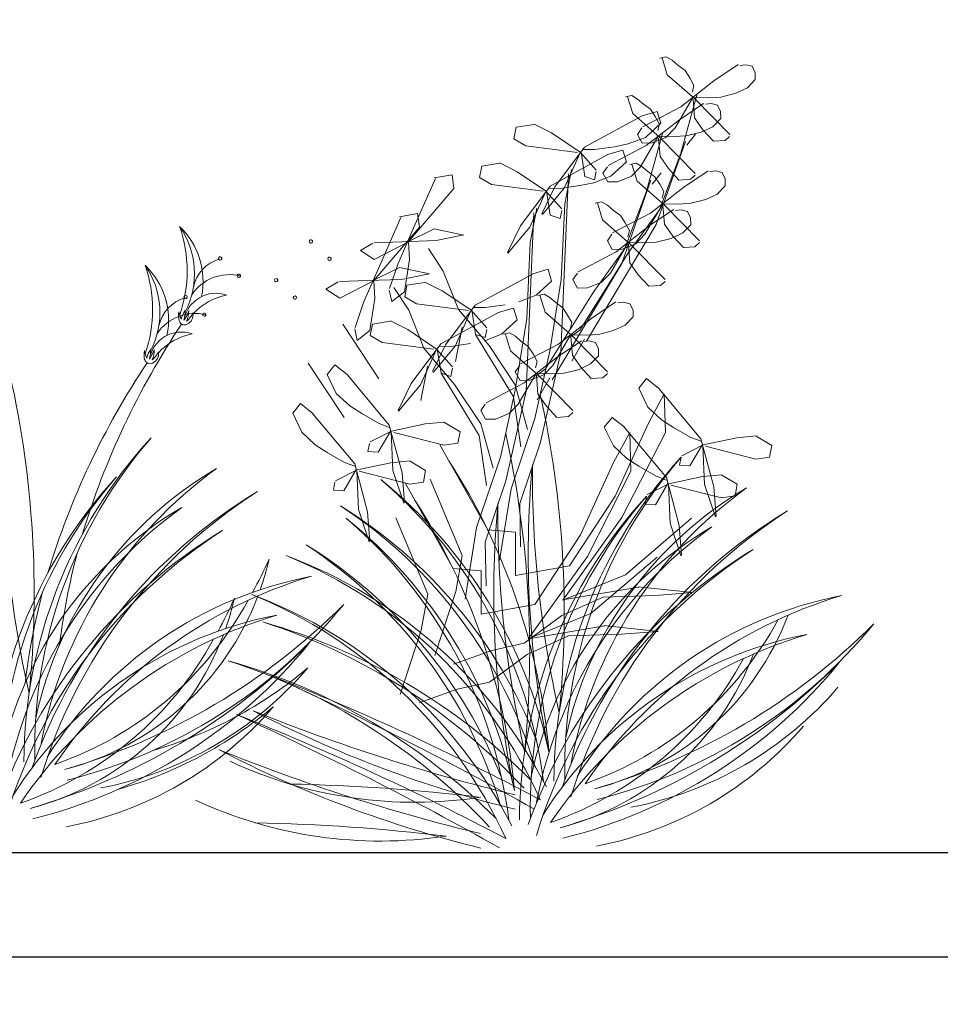
# Model space of a CAD drawing. Units: inches. Extents: x 89 to 490, y -59 to 378.
# Tile 14 of 20: x 400 to 429, y -28 to 3. Entities that reach past the tile are written whole.
import ezdxf

# ---------------------------------------------------------------- set-up
doc = ezdxf.new("R2010")
doc.units = ezdxf.units.IN
doc.header["$MEASUREMENT"] = 0
for name, color, linetype, lineweight in [('A-ANNO-DIMS', 2, 'Continuous', 18), ('L-PLNT', 94, 'Continuous', 18), ('L-PLNT-EDGE', 31, 'Continuous', 25)]:
    doc.layers.add(name, color=color, linetype=linetype, lineweight=lineweight)
doc.layers.add('fl', color=73, linetype='Continuous', lineweight=9, true_color=0xa3d166)
doc.styles.get("Standard").update_dxf_attribs({"font": 'arial.ttf'})
doc.dimstyles.get("Standard").update_dxf_attribs({"dimtxt": 6, "dimasz": 4, "dimexe": 3, "dimexo": 3, "dimgap": 0.09, "dimtad": 0, "dimtih": 1, "dimtoh": 1, "dimdec": 1, "dimzin": 0, "dimdsep": 46, "dimlunit": 3, "dimtxsty": 'Standard', "dimcen": 0.09, "dimadec": 0, "dimazin": 0, "dimtfac": 1, "dimtdec": 1, "dimtofl": 0, "dimtmove": 0, "dimatfit": 3, "dimfxl": 1, "dimtolj": 1, "dimtzin": 0, "dimarcsym": 0})

# ---------------------------------------------------------------- blocks, each defined once
blk = doc.blocks.new('Plantation')
at = {"layer": 'fl'}
for p, q in [((644.446, 36.432), (644.645, 36.472)), ((644.513, 36.439), (644.677, 35.91)), ((644.645, 36.472), (644.829, 36.366)), ((644.829, 36.366), (645.013, 36.206)), ((645.013, 36.206), (645.235, 36.046)), ((646.142, 35.717), (646.902, 36.229)), ((647.142, 36.225), (646.96, 36.203)), ((647.343, 36.174), (647.142, 36.225)), ((647.437, 35.975), (647.343, 36.174)), ((644.677, 35.91), (645.529, 35.161)), ((645.235, 36.046), (645.384, 35.812)), ((647.441, 35.756), (647.437, 35.975)), ((645.1, 34.903), (646.142, 35.717)), ((645.384, 35.812), (645.516, 35.577)), ((645.516, 35.577), (645.465, 35.376)), ((647.191, 35.497), (647.441, 35.756)), ((643.362, 35.214), (643.561, 35.254)), ((643.561, 35.254), (643.745, 35.148)), ((645.101, 33.445), (645.621, 35.31)), ((646.359, 35.209), (646.83, 35.327)), ((646.83, 35.327), (647.191, 35.497)), ((643.429, 35.221), (643.593, 34.692)), ((643.745, 35.148), (643.93, 34.988)), ((643.93, 34.988), (644.151, 34.828)), ((644.921, 34.238), (645.468, 35.176)), ((645.058, 34.499), (645.818, 35.011)), ((645.487, 35.14), (645.533, 34.558)), ((645.522, 35.195), (645.977, 35.185)), ((645.529, 35.161), (646.637, 34.032)), ((646.058, 35.007), (645.876, 34.985)), ((645.977, 35.185), (646.359, 35.209)), ((646.259, 34.955), (646.058, 35.007)), ((646.353, 34.757), (646.259, 34.955)), ((643.593, 34.692), (644.445, 33.943)), ((644.364, 34.761), (643.889, 34.62)), ((643.906, 34.279), (645.1, 34.903)), ((644.151, 34.828), (644.3, 34.594)), ((644.477, 34.391), (644.364, 34.761)), ((646.357, 34.538), (646.353, 34.757)), ((640.494, 34.348), (639.938, 34.259)), ((640.5, 34.358), (641.044, 34.084)), ((642.081, 33.634), (643.894, 34.619)), ((643.994, 33.944), (644.477, 34.391)), ((644.016, 33.685), (645.058, 34.499)), ((644.3, 34.594), (644.432, 34.359)), ((644.432, 34.359), (644.381, 34.158)), ((645.533, 34.558), (645.795, 34.18)), ((646.107, 34.279), (646.357, 34.538)), ((639.938, 34.259), (639.865, 33.899)), ((641.044, 34.084), (641.94, 33.483)), ((643.884, 34.238), (643.742, 34.035)), ((643.742, 34.035), (643.892, 33.764)), ((644.017, 32.227), (644.537, 34.092)), ((644.635, 33.941), (644.921, 34.238)), ((645.275, 33.991), (645.746, 34.109)), ((645.287, 33.694), (645.567, 34.044)), ((645.746, 34.109), (646.107, 34.279)), ((645.795, 34.18), (646.128, 33.822)), ((639.865, 33.899), (640.24, 33.679)), ((643.016, 33.648), (643.453, 33.736)), ((643.453, 33.736), (643.994, 33.944)), ((643.837, 33.02), (644.384, 33.958)), ((643.892, 33.764), (644.201, 33.77)), ((644.201, 33.77), (644.635, 33.941)), ((644.334, 31.205), (645.245, 33.818)), ((644.403, 33.922), (644.45, 33.34)), ((644.438, 33.977), (644.893, 33.967)), ((644.445, 33.943), (645.553, 32.814)), ((644.893, 33.967), (645.275, 33.991)), ((646.128, 33.822), (646.492, 33.846)), ((646.492, 33.846), (646.635, 33.976)), ((640.24, 33.679), (641.864, 33.469)), ((640.997, 32.416), (642.81, 33.401)), ((641.151, 32.387), (642.081, 33.634)), ((641.445, 32.345), (641.944, 33.457)), ((641.94, 33.483), (642.445, 32.917)), ((642.09, 32.715), (641.97, 33.484)), ((642.048, 33.565), (642.394, 33.558)), ((642.394, 33.558), (643.016, 33.648)), ((643.281, 33.543), (642.805, 33.402)), ((642.822, 33.061), (644.016, 33.685)), ((643.393, 33.173), (643.281, 33.543)), ((644.432, 31.672), (645.101, 33.445)), ((639.41, 33.13), (638.854, 33.041)), ((639.417, 33.139), (639.961, 32.866)), ((642.91, 32.726), (643.393, 33.173)), ((643.501, 33.096), (643.701, 33.136)), ((643.568, 33.102), (643.732, 32.573)), ((643.701, 33.136), (643.884, 33.03)), ((644.45, 33.34), (644.711, 32.962)), ((637.356, 32.671), (637.92, 32.769)), ((637.92, 32.769), (637.978, 32.343)), ((638.854, 33.041), (638.781, 32.681)), ((639.961, 32.866), (640.856, 32.265)), ((641.575, 32.797), (641.331, 27.189)), ((641.46, 31.862), (641.667, 32.939)), ((642.446, 32.868), (642.397, 32.614)), ((642.8, 33.02), (642.658, 32.817)), ((642.658, 32.817), (642.808, 32.546)), ((643.551, 32.723), (643.837, 33.02)), ((643.884, 33.03), (644.069, 32.869)), ((644.069, 32.869), (644.29, 32.709)), ((644.203, 32.476), (644.483, 32.826)), ((644.711, 32.962), (645.045, 32.604)), ((645.197, 32.38), (645.958, 32.892)), ((646.197, 32.888), (646.016, 32.867)), ((646.398, 32.837), (646.197, 32.888)), ((646.493, 32.638), (646.398, 32.837)), ((636.767, 31.216), (637.399, 32.648)), ((638.781, 32.681), (639.157, 32.461)), ((639.157, 32.461), (640.78, 32.251)), ((641.932, 32.43), (642.369, 32.518)), ((642.397, 32.614), (642.09, 32.715)), ((642.369, 32.518), (642.91, 32.726)), ((642.808, 32.546), (643.117, 32.552)), ((643.117, 32.552), (643.551, 32.723)), ((643.25, 29.987), (644.161, 32.6)), ((643.732, 32.573), (644.584, 31.824)), ((644.29, 32.709), (644.44, 32.475)), ((644.44, 32.475), (644.571, 32.24)), ((645.045, 32.604), (645.408, 32.628)), ((645.408, 32.628), (645.551, 32.758)), ((646.497, 32.42), (646.493, 32.638)), ((637.978, 32.343), (636.549, 30.67)), ((640.067, 31.169), (640.997, 32.416)), ((640.362, 31.127), (640.86, 32.239)), ((640.742, 31.546), (641.151, 32.387)), ((640.756, 31.523), (641.445, 32.345)), ((640.856, 32.265), (641.362, 31.699)), ((641.006, 31.497), (640.886, 32.266)), ((640.964, 32.347), (641.31, 32.34)), ((641.31, 32.34), (641.932, 32.43)), ((643.348, 30.454), (644.017, 32.227)), ((644.156, 31.567), (645.197, 32.38)), ((644.571, 32.24), (644.52, 32.039)), ((645.885, 31.99), (646.246, 32.16)), ((646.246, 32.16), (646.497, 32.42)), ((641.347, 29.477), (641.46, 31.862)), ((642.417, 31.878), (642.617, 31.918)), ((642.485, 31.884), (642.648, 31.355)), ((642.617, 31.918), (642.8, 31.812)), ((644.578, 31.858), (645.033, 31.848)), ((645.033, 31.848), (645.415, 31.873)), ((645.415, 31.873), (645.885, 31.99)), ((636.272, 31.453), (636.836, 31.551)), ((636.836, 31.551), (636.894, 31.125)), ((640.491, 31.579), (640.247, 25.971)), ((640.377, 30.644), (640.583, 31.721)), ((641.362, 31.65), (641.313, 31.396)), ((642.8, 31.812), (642.985, 31.651)), ((642.961, 30.943), (644.156, 31.567)), ((642.985, 31.651), (643.206, 31.491)), ((643.457, 30.326), (644.432, 31.672)), ((643.976, 30.901), (644.524, 31.839)), ((644.113, 31.162), (644.874, 31.674)), ((644.542, 31.803), (644.589, 31.221)), ((644.584, 31.824), (645.692, 30.695)), ((645.113, 31.67), (644.932, 31.649)), ((645.314, 31.619), (645.113, 31.67)), ((645.409, 31.42), (645.314, 31.619)), ((635.683, 29.998), (636.315, 31.43)), ((641.313, 31.396), (641.006, 31.497)), ((642.648, 31.355), (643.5, 30.606)), ((643.206, 31.491), (643.356, 31.257)), ((643.356, 31.257), (643.487, 31.022)), ((645.413, 31.202), (645.409, 31.42)), ((636.894, 31.125), (635.465, 29.452)), ((636.226, 29.982), (636.767, 31.216)), ((637.359, 31.074), (636.512, 30.657)), ((638.292, 30.877), (637.359, 31.074)), ((639.658, 30.328), (640.067, 31.169)), ((639.672, 30.305), (640.362, 31.127)), ((642.144, 27.545), (644.334, 31.205)), ((643.072, 30.349), (644.113, 31.162)), ((643.487, 31.022), (643.436, 30.821)), ((644.589, 31.221), (644.85, 30.843)), ((644.802, 30.772), (645.163, 30.942)), ((645.163, 30.942), (645.413, 31.202)), ((635.432, 30.626), (635.046, 30.393)), ((635.474, 30.637), (636.348, 30.667)), ((635.478, 30.111), (636.537, 30.658)), ((636.348, 30.667), (637.417, 30.704)), ((636.584, 30.105), (636.55, 30.658)), ((637.417, 30.704), (638.286, 30.879)), ((640.264, 28.259), (640.377, 30.644)), ((642.939, 30.901), (642.797, 30.698)), ((642.797, 30.698), (642.947, 30.428)), ((642.892, 29.683), (643.44, 30.621)), ((643.494, 30.64), (643.949, 30.63)), ((643.5, 30.606), (644.608, 29.477)), ((643.69, 30.605), (643.976, 30.901)), ((643.949, 30.63), (644.331, 30.655)), ((644.331, 30.655), (644.802, 30.772)), ((644.85, 30.843), (645.184, 30.485)), ((645.547, 30.509), (645.691, 30.639)), ((635.046, 30.393), (635.478, 30.111)), ((637.182, 30.453), (637.644, 29.739)), ((641.878, 29.724), (643.072, 30.349)), ((641.936, 27.892), (643.457, 30.326)), ((642.374, 29.108), (643.348, 30.454)), ((642.947, 30.428), (643.257, 30.433)), ((643.257, 30.433), (643.69, 30.605)), ((643.459, 30.585), (643.505, 30.003)), ((645.184, 30.485), (645.547, 30.509)), ((635.142, 28.764), (635.683, 29.998)), ((636.426, 29.096), (636.584, 30.105)), ((643.505, 30.003), (643.766, 29.625)), ((636.275, 29.856), (635.428, 29.439)), ((635.961, 29.196), (636.226, 29.982)), ((637.208, 29.659), (636.275, 29.856)), ((637.644, 29.739), (638.122, 28.54)), ((640.933, 29.803), (640.457, 29.662)), ((641.045, 29.433), (640.933, 29.803)), ((641.061, 26.327), (643.25, 29.987)), ((641.855, 29.683), (641.713, 29.48)), ((642.606, 29.387), (642.892, 29.683)), ((634.348, 29.408), (633.962, 29.175)), ((634.39, 29.419), (635.264, 29.449)), ((634.395, 28.893), (635.453, 29.44)), ((635.264, 29.449), (636.333, 29.486)), ((635.5, 28.887), (635.466, 29.44)), ((636.333, 29.486), (637.202, 29.661)), ((637.062, 29.39), (636.506, 29.301)), ((637.069, 29.4), (637.613, 29.126)), ((638.649, 28.676), (640.463, 29.661)), ((640.562, 28.986), (641.045, 29.433)), ((640.987, 27.228), (641.347, 29.477)), ((641.713, 29.48), (641.863, 29.21)), ((642.173, 29.215), (642.606, 29.387)), ((643.766, 29.625), (644.1, 29.267)), ((644.464, 29.291), (644.607, 29.421)), ((633.962, 29.175), (634.395, 28.893)), ((635.948, 29.151), (636.029, 28.787)), ((636.029, 28.787), (636.426, 29.096)), ((636.098, 29.235), (636.56, 28.521)), ((636.506, 29.301), (636.433, 28.941)), ((637.613, 29.126), (638.508, 28.525)), ((640.852, 26.674), (642.374, 29.108)), ((641.863, 29.21), (642.173, 29.215)), ((644.1, 29.267), (644.464, 29.291)), ((634.877, 27.978), (635.142, 28.764)), ((635.342, 27.878), (635.5, 28.887)), ((636.433, 28.941), (636.809, 28.721)), ((640.021, 28.778), (640.562, 28.986)), ((640.61, 28.981), (640.809, 29.021)), ((640.677, 28.987), (640.841, 28.458)), ((640.809, 29.021), (640.993, 28.915)), ((640.993, 28.915), (641.178, 28.754)), ((641.178, 28.754), (641.399, 28.594)), ((642.306, 28.265), (643.067, 28.777)), ((643.306, 28.773), (643.125, 28.752)), ((643.507, 28.722), (643.306, 28.773)), ((636.56, 28.521), (637.038, 27.322)), ((636.809, 28.721), (638.432, 28.511)), ((637.565, 27.458), (639.379, 28.443)), ((637.719, 27.429), (638.649, 28.676)), ((638.014, 27.387), (638.512, 28.499)), ((638.122, 28.54), (639.085, 27.406)), ((638.508, 28.525), (639.014, 27.959)), ((638.658, 27.757), (638.538, 28.526)), ((638.616, 28.607), (638.962, 28.6)), ((638.962, 28.6), (639.584, 28.69)), ((639.849, 28.585), (639.373, 28.444)), ((639.961, 28.215), (639.849, 28.585)), ((640.841, 28.458), (641.693, 27.71)), ((641.399, 28.594), (641.549, 28.36)), ((643.602, 28.523), (643.507, 28.722)), ((643.605, 28.305), (643.602, 28.523)), ((635.979, 28.172), (635.422, 28.083)), ((635.985, 28.182), (636.529, 27.908)), ((639.478, 27.768), (639.961, 28.215)), ((639.903, 26.01), (640.264, 28.259)), ((641.264, 27.452), (642.306, 28.265)), ((641.549, 28.36), (641.68, 28.126)), ((643.355, 28.046), (643.605, 28.305)), ((634.492, 28.076), (635.62, 26.364)), ((634.864, 27.933), (634.945, 27.569)), ((634.945, 27.569), (635.342, 27.878)), ((635.422, 28.083), (635.349, 27.723)), ((636.529, 27.908), (637.424, 27.307)), ((638.029, 26.904), (638.235, 27.981)), ((639.014, 27.91), (638.965, 27.656)), ((641.68, 28.126), (641.629, 27.925)), ((641.651, 27.688), (641.936, 27.892)), ((642.523, 27.758), (642.994, 27.876)), ((642.994, 27.876), (643.355, 28.046)), ((635.349, 27.723), (635.725, 27.503)), ((638.658, 27.757), (639.853, 25.796)), ((638.965, 27.656), (638.658, 27.757)), ((638.937, 27.56), (639.478, 27.768)), ((639.526, 27.763), (639.726, 27.803)), ((639.594, 27.769), (639.757, 27.24)), ((639.726, 27.803), (639.909, 27.697)), ((639.909, 27.697), (640.094, 27.536)), ((640.094, 27.536), (640.315, 27.376)), ((641.085, 26.786), (641.633, 27.724)), ((641.222, 27.047), (641.983, 27.559)), ((641.651, 27.688), (641.698, 27.106)), ((641.677, 26.921), (642.075, 27.612)), ((641.687, 27.743), (642.142, 27.733)), ((641.693, 27.71), (642.801, 26.581)), ((642.222, 27.555), (642.041, 27.534)), ((642.142, 27.733), (642.523, 27.758)), ((642.423, 27.504), (642.222, 27.555)), ((635.725, 27.503), (637.348, 27.293)), ((636.635, 26.211), (637.565, 27.458)), ((636.93, 26.169), (637.428, 27.281)), ((637.038, 27.322), (638.001, 26.188)), ((637.31, 26.588), (637.719, 27.429)), ((637.324, 26.565), (638.014, 27.387)), ((637.424, 27.307), (637.93, 26.741)), ((637.574, 26.539), (637.454, 27.308)), ((637.533, 27.389), (637.878, 27.382)), ((637.878, 27.382), (638.501, 27.472)), ((639.085, 27.406), (639.905, 26.17)), ((639.757, 27.24), (640.609, 26.492)), ((640.07, 26.828), (641.264, 27.452)), ((640.315, 27.376), (640.465, 27.142)), ((640.524, 25.122), (640.987, 27.228)), ((642.518, 27.305), (642.423, 27.504)), ((642.522, 27.087), (642.518, 27.305)), ((640.181, 26.234), (641.222, 27.047)), ((640.465, 27.142), (640.596, 26.908)), ((640.596, 26.908), (640.545, 26.707)), ((641.331, 27.189), (640.697, 24.376)), ((641.698, 27.106), (641.959, 26.729)), ((642.271, 26.828), (642.522, 27.087)), ((633.408, 26.858), (634.536, 25.146)), ((634.001, 26.499), (634.242, 26.801)), ((634.242, 26.801), (634.632, 26.495)), ((636.945, 25.686), (637.151, 26.763)), ((637.93, 26.692), (637.881, 26.438)), ((640.048, 26.786), (639.906, 26.583)), ((640.568, 26.47), (640.852, 26.674)), ((640.799, 26.49), (641.085, 26.786)), ((641.44, 26.54), (641.911, 26.658)), ((641.911, 26.658), (642.271, 26.828)), ((641.959, 26.729), (642.293, 26.37)), ((634.285, 25.905), (634.001, 26.499)), ((635.949, 24.911), (634.626, 26.496)), ((637.574, 26.539), (638.769, 24.578)), ((637.881, 26.438), (637.574, 26.539)), ((639.906, 26.583), (640.056, 26.313)), ((640.001, 25.568), (640.549, 26.506)), ((640.056, 26.313), (640.365, 26.318)), ((640.365, 26.318), (640.799, 26.49)), ((640.568, 26.47), (640.614, 25.888)), ((640.593, 25.703), (640.991, 26.394)), ((640.603, 26.525), (641.058, 26.515)), ((640.609, 26.492), (641.717, 25.363)), ((641.058, 26.515), (641.44, 26.54)), ((642.293, 26.37), (642.656, 26.395)), ((642.656, 26.395), (642.8, 26.525)), ((643.785, 26.065), (644.026, 26.368)), ((644.026, 26.368), (644.416, 26.061)), ((636.226, 25.37), (636.635, 26.211)), ((636.24, 25.347), (636.93, 26.169)), ((638.001, 26.188), (638.821, 24.952)), ((638.987, 25.61), (640.181, 26.234)), ((639.44, 23.904), (639.903, 26.01)), ((640.247, 25.971), (639.613, 23.158)), ((639.905, 26.17), (640.292, 24.774)), ((644.07, 25.472), (643.785, 26.065)), ((645.734, 24.478), (644.411, 26.062)), ((634.711, 25.512), (634.285, 25.905)), ((639.853, 25.796), (640.085, 24.228)), ((640.614, 25.888), (640.875, 25.511)), ((644.078, 24.951), (644.581, 25.892)), ((644.581, 25.892), (644.622, 24.678)), ((632.917, 25.281), (633.158, 25.583)), ((633.158, 25.583), (633.548, 25.277)), ((635.085, 25.27), (634.711, 25.512)), ((638.964, 25.568), (638.822, 25.365)), ((638.822, 25.365), (638.972, 25.095)), ((639.715, 25.272), (640.001, 25.568)), ((640.875, 25.511), (641.209, 25.152)), ((644.496, 25.078), (644.07, 25.472)), ((633.201, 24.687), (632.917, 25.281)), ((634.865, 23.693), (633.543, 25.278)), ((635.63, 24.956), (635.085, 25.27)), ((638.972, 25.095), (639.282, 25.1)), ((639.282, 25.1), (639.715, 25.272)), ((639.773, 22.909), (640.524, 25.122)), ((641.209, 25.152), (641.573, 25.177)), ((641.573, 25.177), (641.716, 25.307)), ((642.701, 24.847), (642.943, 25.15)), ((642.943, 25.15), (643.333, 24.843)), ((644.869, 24.836), (644.496, 25.078)), ((635.954, 24.835), (635.63, 24.956)), ((636.353, 23.409), (635.949, 24.911)), ((637.078, 24.948), (636.024, 24.719)), ((637.685, 25.001), (637.078, 24.948)), ((637.687, 24.991), (638.171, 24.703)), ((638.821, 24.952), (639.209, 23.556)), ((642.986, 24.254), (642.701, 24.847)), ((643.038, 22.68), (644.078, 24.951)), ((644.65, 23.26), (643.327, 24.844)), ((645.415, 24.522), (644.869, 24.836)), ((633.627, 24.294), (633.201, 24.687)), ((636.024, 24.719), (635.346, 24.379)), ((635.602, 24.061), (635.997, 24.731)), ((636.064, 23.479), (636.011, 24.696)), ((637.677, 24.275), (636.09, 24.678)), ((638.171, 24.703), (638.107, 24.341)), ((638.769, 24.578), (639.001, 23.01)), ((642.994, 23.733), (643.497, 24.674)), ((644.622, 24.678), (643.255, 22.007)), ((643.497, 24.674), (643.538, 23.46)), ((645.738, 24.402), (645.415, 24.522)), ((646.138, 22.976), (645.734, 24.478)), ((646.863, 24.515), (645.809, 24.286)), ((647.469, 24.568), (646.863, 24.515)), ((647.472, 24.557), (647.956, 24.269)), ((634.001, 24.052), (633.627, 24.294)), ((635.327, 24.334), (635.279, 24.08)), ((637.538, 24.291), (639.039, 21.62)), ((638.107, 24.341), (637.677, 24.275)), ((640.697, 24.376), (640.048, 22.451)), ((643.412, 23.86), (642.986, 24.254)), ((645.809, 24.286), (645.13, 23.946)), ((645.387, 23.627), (645.781, 24.297)), ((645.849, 23.046), (645.796, 24.263)), ((647.461, 23.842), (645.874, 24.244)), ((647.956, 24.269), (647.891, 23.907)), ((634.546, 23.738), (634.001, 24.052)), ((635.279, 24.08), (635.602, 24.061)), ((638.689, 21.691), (639.44, 23.904)), ((643.786, 23.618), (643.412, 23.86)), ((645.112, 23.9), (645.064, 23.647)), ((647.891, 23.907), (647.461, 23.842)), ((634.94, 23.501), (634.262, 23.161)), ((634.518, 22.843), (634.913, 23.513)), ((634.87, 23.617), (634.546, 23.738)), ((635.27, 22.191), (634.865, 23.693)), ((635.995, 23.73), (634.94, 23.501)), ((636.601, 23.783), (635.995, 23.73)), ((636.603, 23.773), (637.087, 23.485)), ((641.954, 21.462), (642.994, 23.733)), ((644.331, 23.304), (643.786, 23.618)), ((645.064, 23.647), (645.387, 23.627)), ((634.981, 22.261), (634.927, 23.478)), ((636.593, 23.057), (635.006, 23.46)), ((636.402, 22.46), (636.064, 23.479)), ((636.424, 22.477), (636.353, 23.409)), ((637.087, 23.485), (637.023, 23.123)), ((638.24, 20.815), (637.235, 23.211)), ((643.538, 23.46), (642.171, 20.789)), ((644.655, 23.184), (644.331, 23.304)), ((645.054, 21.758), (644.65, 23.26)), ((645.779, 23.297), (644.725, 23.068)), ((646.386, 23.35), (645.779, 23.297)), ((646.388, 23.339), (646.872, 23.051)), ((634.244, 23.116), (634.195, 22.862)), ((636.454, 23.073), (637.955, 20.402)), ((637.023, 23.123), (636.593, 23.057)), ((639.613, 23.158), (638.964, 21.233)), ((639.412, 20.66), (639.773, 22.909)), ((644.725, 23.068), (644.047, 22.728)), ((644.303, 22.409), (644.697, 23.079)), ((644.765, 21.828), (644.712, 23.045)), ((646.377, 22.624), (644.79, 23.026)), ((646.187, 22.027), (645.849, 23.046)), ((646.208, 22.044), (646.138, 22.976)), ((646.872, 23.051), (646.807, 22.689)), ((634.195, 22.862), (634.518, 22.843)), ((641.605, 20.492), (643.038, 22.68)), ((644.028, 22.682), (643.98, 22.428)), ((646.807, 22.689), (646.377, 22.624)), ((635.318, 21.242), (634.981, 22.261)), ((640.048, 22.451), (640.072, 21.085)), ((643.98, 22.428), (644.303, 22.409)), ((635.34, 21.259), (635.27, 22.191)), ((637.156, 19.597), (636.151, 21.993)), ((643.255, 22.007), (641.399, 19.415)), ((643.365, 20.212), (645.443, 21.984)), ((638.328, 19.442), (638.689, 21.691)), ((645.103, 20.809), (644.765, 21.828)), ((645.125, 20.826), (645.054, 21.758)), ((639.039, 21.62), (639.916, 21.552)), ((639.916, 21.552), (639.914, 20.191)), ((640.521, 19.274), (641.954, 21.462)), ((638.964, 21.233), (638.988, 19.867)), ((638.035, 19.69), (638.24, 20.815)), ((642.171, 20.789), (640.315, 18.197)), ((642.281, 18.994), (644.359, 20.766)), ((639.914, 20.191), (641.605, 20.492)), ((637.955, 20.402), (638.832, 20.334)), ((638.832, 20.334), (638.83, 18.973)), ((641.399, 19.415), (643.365, 20.212)), ((643.787, 19.825), (641.4, 19.421)), ((643.766, 19.836), (645.474, 19.652)), ((636.951, 18.472), (637.156, 19.597)), ((637.375, 17.674), (638.035, 19.69)), ((642.66, 19.507), (641.367, 18.928)), ((644.311, 19.563), (642.66, 19.507)), ((645.474, 19.652), (644.311, 19.563)), ((638.83, 18.973), (640.521, 19.274)), ((641.367, 18.928), (640.181, 18.061)), ((640.315, 18.197), (642.281, 18.994)), ((642.704, 18.607), (640.316, 18.203)), ((642.683, 18.618), (644.39, 18.434)), ((636.291, 16.456), (636.951, 18.472)), ((641.576, 18.289), (640.283, 17.71)), ((643.227, 18.345), (641.576, 18.289)), ((644.39, 18.434), (643.227, 18.345)), ((640.181, 18.061), (639.168, 17.832)), ((639.168, 17.832), (637.967, 17.403)), ((640.283, 17.71), (639.097, 16.843)), ((639.097, 16.843), (638.084, 16.614)), ((638.084, 16.614), (636.883, 16.185))]:
    blk.add_line(p, q, dxfattribs=at)
for centre, radius, start, end in [((627.233, 29.66), 2.601, 332.7126, 34.904), ((627.729, 29.428), 2.375, 348.2707, 46.4368), ((625.377, 29.751), 4.227, 340.8803, 19.3142), ((633.485, 30.675), 0.053, 350.198, 170.198), ((633.485, 30.675), 0.053, 170.198, 350.198), ((630.941, 29.008), 1.163, 105.8563, 168.2872), ((630.64, 30.141), 0.053, 170.198, 350.198), ((630.64, 30.141), 0.053, 350.198, 170.198), ((634.072, 30.129), 0.053, 170.198, 350.198), ((634.072, 30.129), 0.053, 350.198, 170.198), ((626.149, 28.442), 2.601, 332.7126, 34.904), ((626.645, 28.209), 2.375, 348.2707, 46.4368), ((624.293, 28.533), 4.227, 340.8803, 19.3142), ((630.928, 28.217), 1.416, 75.596, 146.3364), ((631.228, 29.595), 0.053, 350.198, 170.198), ((631.228, 29.595), 0.053, 170.198, 350.198), ((632.401, 29.457), 0.053, 170.198, 350.198), ((632.401, 29.457), 0.053, 350.198, 170.198), ((629.858, 27.79), 1.163, 105.8563, 168.2872), ((629.556, 28.923), 0.053, 170.198, 350.198), ((630.502, 28.038), 1.01, 70.2507, 170.8138), ((629.556, 28.923), 0.053, 350.198, 170.198), ((631.191, 27.136), 1.886, 100.6373, 137.9791), ((632.989, 28.911), 0.053, 350.198, 170.198), ((632.989, 28.911), 0.053, 170.198, 350.198), ((630.022, 28.346), 0.688, 169.5666, 193.8466), ((630.536, 28.704), 1.213, 191.1134, 202.9272), ((630.196, 28.033), 0.803, 144.0451, 165.6539), ((628.034, 28.557), 1.513, 346.3307, 357.9859), ((628.834, 28.719), 0.848, 322.2492, 344.6889), ((628.999, 28.458), 0.654, 334.2428, 3.277), ((629.844, 26.999), 1.416, 75.596, 146.3364), ((629.522, 28.231), 0.175, 196.6761, 296.6412), ((629.155, 28.71), 0.689, 308.8656, 336.2578), ((629.457, 28.377), 0.334, 295.3934, 9.6219), ((630.144, 28.377), 0.053, 170.198, 350.198), ((630.144, 28.377), 0.053, 350.198, 170.198), ((649.959, 14.352), 24.696, 146.2244, 163.2125), ((629.418, 26.82), 1.01, 70.2507, 170.8138), ((630.107, 25.918), 1.886, 100.6373, 137.9791), ((628.938, 27.128), 0.688, 169.5666, 193.8466), ((629.452, 27.486), 1.213, 191.1134, 202.9272), ((629.112, 26.815), 0.803, 144.0451, 165.6539), ((626.95, 27.339), 1.513, 346.3307, 357.9859), ((627.75, 27.501), 0.848, 322.2492, 344.6889), ((627.915, 27.24), 0.654, 334.2428, 3.277), ((628.071, 27.492), 0.689, 308.8656, 336.2578), ((628.373, 27.159), 0.334, 295.3934, 9.6219), ((628.438, 27.013), 0.175, 196.6761, 296.6412), ((648.875, 13.134), 24.696, 146.2244, 163.2125), ((593.308, 19.626), 31.492, 354.2791, 12.5427), ((609.95, 19.019), 31.492, 354.2791, 12.5427), ((639.676, 14.236), 15.201, 137.4916, 179.6099), ((639.738, 14.726), 14.921, 139.0392, 181.297), ((608.866, 17.801), 31.492, 354.2791, 12.5427), ((657.789, 24.006), 33.989, 179.5471, 192.7817), ((656.318, 13.629), 15.201, 137.4916, 179.6099), ((656.38, 14.119), 14.921, 139.0392, 181.297), ((636.596, 13.174), 12.017, 120.3536, 167.8423), ((638.625, 12.302), 13.856, 125.7805, 169.1581), ((620.829, 12.838), 20.216, 5.151, 32.7872), ((670.206, 20.863), 29.894, 174.6174, 191.9895), ((674.431, 23.399), 33.989, 179.5471, 192.7817), ((638.593, 13.018), 15.201, 137.4916, 179.6099), ((638.654, 13.508), 14.921, 139.0392, 181.297), ((625.984, 11.862), 14.921, 7.1968, 49.4547), ((626.118, 11.386), 15.201, 12.4122, 51.0023), ((653.238, 12.566), 12.017, 120.3536, 167.8423), ((655.267, 11.695), 13.856, 125.7805, 169.1581), ((640.42, 8.581), 16.642, 121.1471, 160.292), ((640.553, 9.138), 16.239, 122.567, 163.1344), ((619.745, 11.62), 20.216, 5.151, 32.7872), ((655.234, 12.411), 15.201, 137.4916, 179.6099), ((655.296, 12.901), 14.921, 139.0392, 181.297), ((635.513, 11.956), 12.017, 120.3536, 167.8423), ((637.541, 11.084), 13.856, 125.7805, 169.1581), ((626.236, 9.896), 14.921, 16.8321, 56.7339), ((626.428, 9.441), 15.201, 21.5651, 58.2814), ((669.122, 19.645), 29.894, 174.6174, 191.9895), ((673.347, 22.181), 33.989, 179.5471, 192.7817), ((624.901, 10.644), 14.921, 7.1968, 49.4547), ((625.034, 10.168), 15.201, 12.4122, 51.0023), ((657.061, 7.974), 16.642, 121.1471, 160.292), ((657.195, 8.531), 16.239, 122.567, 163.1344), ((652.154, 11.348), 12.017, 120.3536, 167.8423), ((654.183, 10.477), 13.856, 125.7805, 169.1581), ((639.336, 7.363), 16.642, 121.1471, 160.292), ((639.469, 7.92), 16.239, 122.567, 163.1344), ((625.152, 8.678), 14.921, 16.8321, 56.7339), ((625.345, 8.223), 15.201, 21.5651, 58.2814), ((647.497, 15.299), 22.067, 165.3183, 172.932), ((627.373, 6.58), 15.201, 27.2807, 69.4256), ((627.097, 6.989), 14.921, 24.3637, 67.878), ((655.978, 6.756), 16.642, 121.1471, 160.292), ((656.111, 7.313), 16.239, 122.567, 163.1344), ((620.304, 25.94), 12.977, 331.0459, 336.1667), ((623.521, 22.688), 8.88, 340.6151, 347.0426), ((635.909, 7.754), 12.64, 100.96, 147.8088), ((637.792, 5.882), 14.911, 106.7083, 145.8338), ((646.413, 14.081), 22.067, 165.3183, 172.932), ((623.521, 22.688), 8.88, 284.6053, 339.2893), ((619.22, 24.722), 12.977, 331.0459, 336.1667), ((622.437, 21.47), 8.88, 340.6151, 347.0426), ((626.29, 5.362), 15.201, 27.2807, 69.4256), ((626.013, 5.771), 14.921, 24.3637, 67.878), ((652.55, 7.146), 12.64, 100.96, 147.8088), ((654.434, 5.275), 14.911, 106.7083, 145.8338), ((621.815, 24.681), 11.042, 289.2472, 331.4766), ((620.045, 33.747), 20.466, 286.2137, 315.0057), ((621.871, 29.597), 16.324, 284.0723, 320.7861), ((634.825, 6.536), 12.64, 100.96, 147.8088), ((636.709, 4.664), 14.911, 106.7083, 145.8338), ((640.162, 22.08), 8.88, 284.6053, 339.2893), ((626.755, 0.259), 19.194, 44.7494, 74.2143), ((626.133, 0.496), 19.147, 42.8064, 72.2288), ((638.457, 24.074), 11.042, 289.2472, 331.4766), ((636.687, 33.14), 20.466, 286.2137, 315.0057), ((638.512, 28.99), 16.324, 284.0723, 320.7861), ((622.437, 21.47), 8.88, 284.6053, 339.2893), ((651.466, 5.928), 12.64, 100.96, 147.8088), ((653.35, 4.057), 14.911, 106.7083, 145.8338), ((620.731, 23.463), 11.042, 289.2472, 331.4766), ((618.961, 32.529), 20.466, 286.2137, 315.0057), ((620.787, 28.379), 16.324, 284.0723, 320.7861), ((639.078, 20.862), 8.88, 284.6053, 339.2893), ((625.672, -0.959), 19.194, 44.7494, 74.2143), ((625.049, -0.722), 19.147, 42.8064, 72.2288), ((637.373, 22.856), 11.042, 289.2472, 331.4766), ((635.603, 31.922), 20.466, 286.2137, 315.0057), ((637.429, 27.772), 16.324, 284.0723, 320.7861), ((624.784, 24.645), 11.325, 280.7497, 319.4803), ((624.921, 27.326), 13.137, 285.9859, 310.1616), ((587.709, -81.018), 107.696, 60.65352, 65.57668), ((601.843, -59.986), 82.807, 62.02355, 68.46556), ((641.426, 24.037), 11.325, 280.7497, 319.4803), ((623.7, 23.427), 11.325, 280.7497, 319.4803), ((623.837, 26.108), 13.137, 285.9859, 310.1616), ((586.625, -82.236), 107.696, 60.65352, 65.57668), ((600.759, -61.204), 82.807, 62.02355, 68.46556), ((648.641, 48.565), 36.77, 242.5259, 256.2554), ((653.628, 70.211), 58.541, 247.9781, 256.44), ((640.342, 22.819), 11.325, 280.7497, 319.4803), ((647.558, 47.347), 36.77, 242.5259, 256.2554), ((652.544, 68.993), 58.541, 247.9781, 256.44), ((636.747, 26.772), 13.704, 244.9915, 278.6666), ((631.625, -46.704), 60.356, 83.15791, 88.86091), ((635.663, 25.554), 13.704, 244.9915, 278.6666), ((630.542, -47.922), 60.356, 83.15791, 88.86091)]:
    blk.add_arc(centre, radius, start, end, dxfattribs=at)
blk = doc.blocks.new('*D46')
at = {"layer": 'A-ANNO-DIMS', "color": 0, "lineweight": -2, "transparency": 16777216}
for p, q in [((277.443, -27.866), (277.443, -53.11)), ((445.739, -27.866), (445.739, -53.11)), ((281.443, -50.11), (332.892, -50.11)), ((441.739, -50.11), (390.289, -50.11))]:
    blk.add_line(p, q, dxfattribs=at)
at = {"layer": 'A-ANNO-DIMS', "color": 0, "transparency": 16777216}
for points in [[(281.443, -49.443), (281.443, -50.777), (277.443, -50.11)], [(441.739, -49.443), (441.739, -50.777), (445.739, -50.11)]]:
    blk.add_solid(points, dxfattribs=at)
at = {"layer": 'Defpoints', "color": 0, "transparency": 16777216}
for p in [(277.443, -24.866), (445.739, -24.866), (445.739, -50.11)]:
    blk.add_point(p, dxfattribs=at)
at = {"layer": 'A-ANNO-DIMS', "color": 0, "transparency": 16777216, "insert": (361.591, -50.11), "char_height": 6, "attachment_point": 5}
blk.add_mtext('\\A1;PLANTING 168', dxfattribs=at)
blk = doc.blocks.new('*D48')
at = {"layer": 'A-ANNO-DIMS', "color": 0, "lineweight": -2, "transparency": 16777216}
for p, q in [((127.441, 10.741), (127.441, -49.809)), ((459.441, -29.659), (459.441, -49.809)), ((131.441, -46.809), (286.756, -46.809)), ((455.441, -46.809), (300.127, -46.809))]:
    blk.add_line(p, q, dxfattribs=at)
at = {"layer": 'A-ANNO-DIMS', "color": 0, "transparency": 16777216}
for points in [[(131.441, -46.143), (131.441, -47.476), (127.441, -46.809)], [(455.441, -46.143), (455.441, -47.476), (459.441, -46.809)]]:
    blk.add_solid(points, dxfattribs=at)
at = {"layer": 'Defpoints', "color": 0, "transparency": 16777216}
for p in [(127.441, 13.741), (459.441, -26.659), (459.441, -46.809)]:
    blk.add_point(p, dxfattribs=at)
at = {"layer": 'A-ANNO-DIMS', "color": 0, "transparency": 16777216, "insert": (293.441, -46.809), "char_height": 6, "attachment_point": 5}
blk.add_mtext('\\A1;332', dxfattribs=at)

msp = doc.modelspace()

# ---------------------------------------------------------------- linework, layer by layer
at = {"layer": 'L-PLNT-EDGE'}
for p, q in [((459.4414, -23.3886), (265.4414, -23.3886)), ((459.4414, -26.6594), (265.4414, -26.6594))]:
    msp.add_line(p, q, dxfattribs=at)

# ---------------------------------------------------------------- block references
at = {"layer": 'L-PLNT'}
msp.add_blockref('Plantation', (-223.8856, -34.8668), dxfattribs=at)

# ---------------------------------------------------------------- dimensions: what is measured, and where the dimension line sits
at = {"layer": 'A-ANNO-DIMS'}
dim = msp.add_linear_dim(base=(459.4414, -46.8094), p1=(127.4414, 13.7413), p2=(459.4414, -26.6594), dimstyle='Standard', override={"dimdec": 0, "dimlfac": 1, "dimrnd": 0, "dimzin": 0, "dimdsep": 46, "dimlunit": 2}, dxfattribs=at)
dim.commit()
dim.dimension.update_dxf_attribs({"geometry": '*D48', "text_midpoint": (293.4414, -46.8094)})
dim = msp.add_linear_dim(base=(445.7386, -50.11), p1=(277.443, -24.8656), p2=(445.7386, -24.8656), text='PLANTING <>', dimstyle='Standard', override={"dimdec": 0, "dimlfac": 1, "dimrnd": 0, "dimzin": 0, "dimdsep": 46, "dimlunit": 2}, dxfattribs=at)
dim.commit()
dim.dimension.update_dxf_attribs({"geometry": '*D46', "text_midpoint": (361.5908, -50.11)})

doc.saveas('drawing.dxf')
